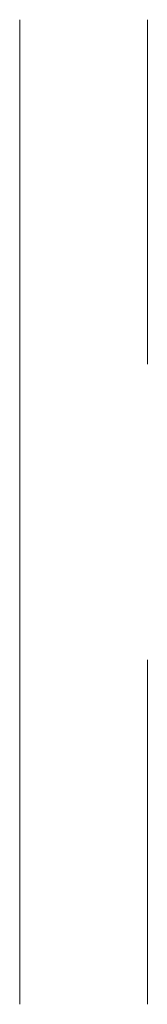
# Model space of a CAD drawing. Units: millimetres. Extents: x 410 to 423, y 261 to 361.
import ezdxf

# ---------------------------------------------------------------- set-up
doc = ezdxf.new("R2010")
doc.units = ezdxf.units.MM
doc.layers.add('M-CONS', color=8, linetype='Continuous', lineweight=13)

msp = doc.modelspace()

# ---------------------------------------------------------------- linework, layer by layer
at = {"layer": 'M-CONS'}
for p, q in [((409.56, 361.27, 125.04), (409.56, 261.27, 125.04)), ((422.56, 326.27, 69.04), (422.56, 361.27, 108.04)), ((409.56, 261.27, 125.04), (409.56, 311.27, 125.04)), ((409.56, 311.27, 125.04), (409.56, 311.27, 135.04)), ((422.56, 296.27, 69.04), (422.56, 261.27, 108.04))]:
    msp.add_line(p, q, dxfattribs=at)

doc.saveas('drawing.dxf')
